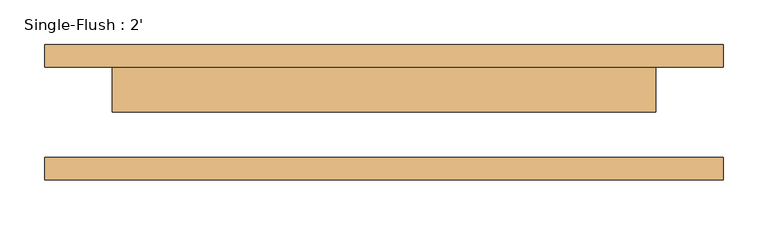
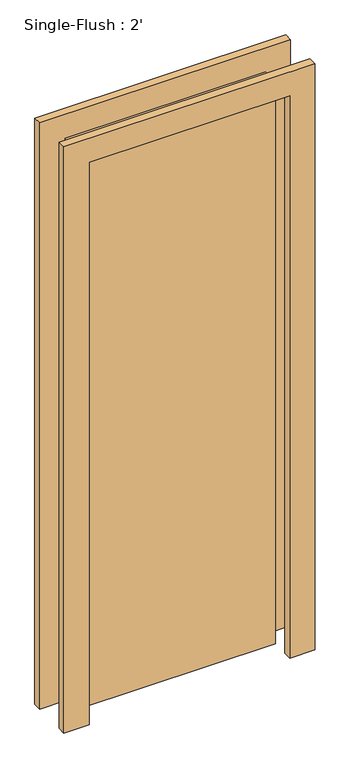
"""IFC4 building model written with IfcOpenShell, lengths in millimetres: door geometry, Single-Flush : 2'."""

from ifc_helpers import new_model, si_unit, frame, origin, origin_with_axes, place, context, project, spatial, polyline, outline, extrude, source, transform, mapped, element, save


def single_flush_2_f3cad073(model_context):
    return source(origin(), model_context, "Body", "SweptSolid", [
        extrude(outline(polyline([(1879.6, -381.0), (0.0, -381.0), (0.0, -304.8), (1803.4, -304.8), (1803.4, 304.8), (0.0, 304.8), (0.0, 381.0), (1879.6, 381.0), (1879.6, -381.0)])), frame((0.0, 50.8, 0.0), z_axis=(0.0, 1.0, 0.0), x_axis=(0.0, 0.0, 1.0)), (0.0, 0.0, 1.0), 25.4),
        extrude(outline(polyline([(1879.6, 381.0), (1879.6, -381.0), (0.0, -381.0), (0.0, -304.8), (1803.4, -304.8), (1803.4, 304.8), (0.0, 304.8), (0.0, 381.0), (1879.6, 381.0)])), frame((0.0, -76.2, 0.0), z_axis=(0.0, 1.0, 0.0), x_axis=(0.0, 0.0, 1.0)), (0.0, 0.0, 1.0), 25.4),
        extrude(outline(polyline([(304.8, 0.0), (-304.8, 0.0), (-304.8, 50.8), (304.8, 50.8), (304.8, 0.0)])), origin_with_axes(), (0.0, 0.0, 1.0), 1803.4),
    ])


if __name__ == "__main__":
    model = new_model("IFC4")
    model_context = context("Model", 3, world=origin())
    ifc_project = project(units=[si_unit("LENGTHUNIT", "METRE", prefix="MILLI")], contexts=[model_context])
    site = spatial("IfcSite", under=ifc_project)
    building = spatial("IfcBuilding", under=site)
    placement = place(None, origin())
    single_flush_2_shape = single_flush_2_f3cad073(model_context)
    element("IfcDoor", 1, ObjectType="Single-Flush : 2'", at=placement, inside=building, context=model_context, shape_type="MappedRepresentation", body=[
        mapped(single_flush_2_shape, transform((0.0, 0.0, 0.0), x_axis=(1.0, 0.0, 0.0), y_axis=(0.0, 1.0, 0.0), z_axis=(0.0, 0.0, 1.0))),
    ])
    save(model, "model.ifc")

# Revit data of these elements
# Type "Single-Flush : 2'"
#   Type Mark = "12"
#   Construction Type Id = "MDOOR"
#   Assembly Code = "C1020"
#   Analytic Construction = "Metal"
#   Thickness = 0' - 2"
#   Heat Transfer Coefficient (U) = 0.651978 BTU/(h·ft²·°F)
#   Height = 5' - 11"
#   Trim Projection Ext = 0' - 1"
#   Trim Projection Int = 0' - 1"
#   Trim Width = 0' - 3"
#   Width = 2' - 0"
#   Define Thermal Properties by = 1
#   Door Material = Door - Panel
#   Frame Material = Door - Frame
#   Visual Light Transmittance = 0
#   Solar Heat Gain Coefficient = 0
#   Function = (empty or 0)
#   Wall Closure = (empty or 0)
# Element 1 (IfcDoor, "Single-Flush : 2'")
#   Materials on its faces: "Door - Frame", "Door - Panel"
# Materials
#   "Door - Panel": class "Wood", colour RGB 210 159 95, transparency 0
#   "Door - Frame": colour RGB 118 70 51, transparency 0
